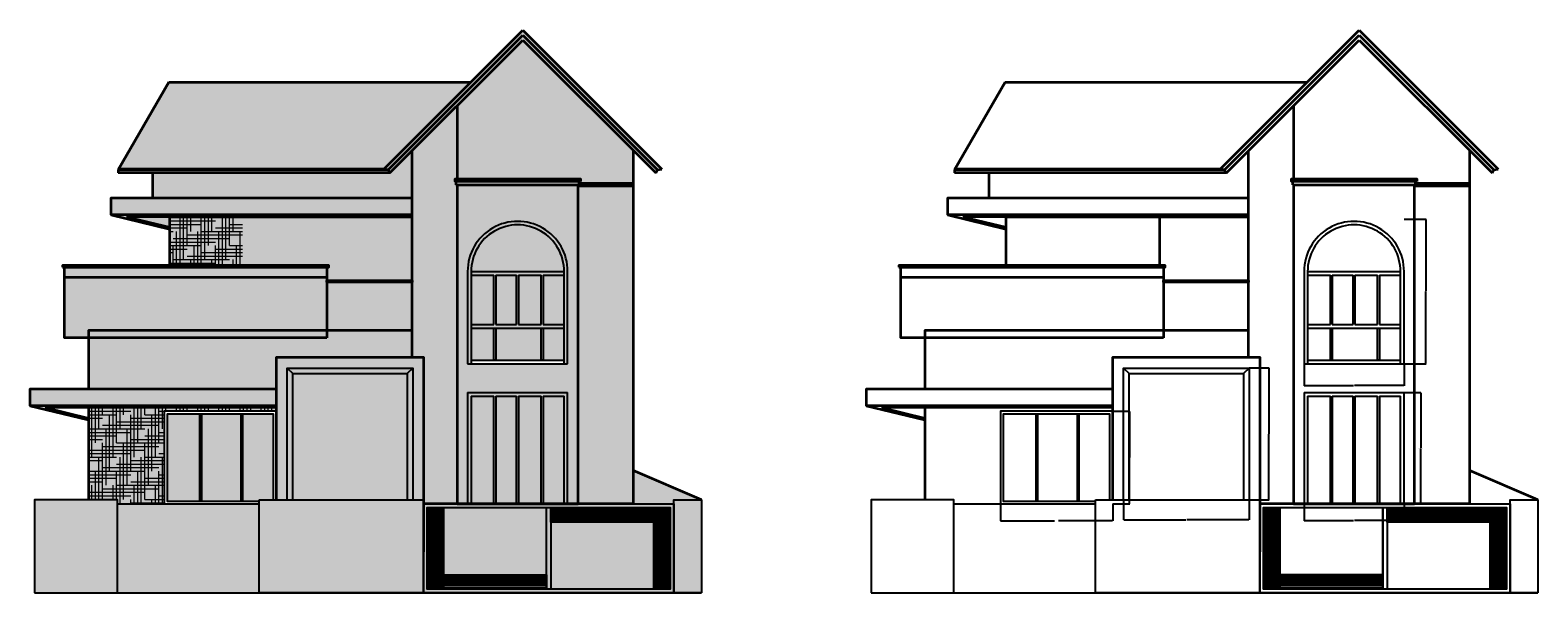
# Model space of a CAD drawing. Units: feet. Extents: x 2649 to 4006, y 754 to 1261.
import ezdxf

# ---------------------------------------------------------------- set-up
doc = ezdxf.new("R2010")
doc.units = ezdxf.units.FT
for name, color, linetype, lineweight in [('A-ANNO-DIMS', 2, 'Continuous', 18), ('A-DOOR', 3, 'Continuous', 25), ('A-ELEV', 7, 'Continuous', 35), ('A-ELEV-FENC', 8, 'Continuous', 25), ('A-ELEV-PATT', 8, 'Continuous', 13), ('A-GLAZ', 4, 'Continuous', 25), ('A-ROOF', 1, 'Continuous', 35)]:
    doc.layers.add(name, color=color, linetype=linetype, lineweight=lineweight)
doc.styles.get("Standard").update_dxf_attribs({"font": 'arial.ttf'})
doc.dimstyles.get("Standard").update_dxf_attribs({"dimtxt": 0.18, "dimasz": 0.18, "dimexe": 0.18, "dimexo": 0.0625, "dimgap": 0.09, "dimtad": 0, "dimtih": 1, "dimtoh": 1, "dimdec": 1, "dimzin": 0, "dimdsep": 46, "dimlunit": 3, "dimtxsty": 'Standard', "dimcen": 0.09, "dimadec": 0, "dimazin": 0, "dimtfac": 1, "dimtdec": 1, "dimtofl": 0, "dimtmove": 0, "dimatfit": 3, "dimfxl": 1, "dimtolj": 1, "dimtzin": 0, "dimarcsym": 0})

# ---------------------------------------------------------------- blocks, each defined once
blk = doc.blocks.new('WIN-ARCHED')
for p, q in [((3.2, 83.1), (86.8, 83.1)), ((3.2, 79.9), (23.7, 79.9)), ((25.4, 79.9), (44.1, 79.9)), ((45.8, 79.9), (66.2, 79.9)), ((67.9, 79.9), (86.8, 79.9)), ((3.2, 35.3), (23.7, 35.3)), ((3.2, 32.1), (86.8, 32.1)), ((25.4, 35.3), (44.1, 35.3)), ((45.8, 35.3), (66.2, 35.3)), ((67.9, 35.3), (86.8, 35.3)), ((0, 0), (90, 0)), ((3.2, 3.2), (86.8, 3.2))]:
    blk.add_line(p, q)
for points in [[(0, 83.4), (0, 0)], [(3.2, 83.5), (3.2, 0)], [(86.8, 0), (86.8, 83.5)], [(90, 0), (90, 83.4)], [(23.7, 35.3), (23.7, 79.9)], [(25.4, 79.9), (25.4, 35.3)], [(44.1, 35.3), (44.1, 79.9)], [(45.8, 79.9), (45.8, 35.3)], [(66.2, 35.3), (66.2, 79.9)], [(67.9, 79.9), (67.9, 35.3)], [(25.4, 32.1), (25.4, 3.2), (23.7, 3.2), (23.7, 32.1)], [(67.9, 32.1), (67.9, 3.2), (66.2, 3.2), (66.2, 32.1)]]:
    blk.add_lwpolyline(points)
for radius, start, end in [(45, 359.816, 180.184), (41.8, 359.7048, 180.2952)]:
    blk.add_arc((45, 83.3), radius, start, end)
blk = doc.blocks.new('DOOR-GLAZED-FRENCH')
for points in [[(0, 100.3), (90, 100.3)], [(0, 100.3), (0, 0)], [(3.2, 97.1), (3.2, 0)], [(3.2, 97.1), (23.7, 97.1)], [(25.4, 97.1), (25.4, 0), (23.7, 0), (23.7, 97.1)], [(25.4, 97.1), (44.1, 97.1)], [(45.8, 97.1), (45.8, 0), (44.1, 0), (44.1, 97.1)], [(45.8, 97.1), (66.2, 97.1)], [(67.9, 97.1), (67.9, 0), (66.2, 0), (66.2, 97.1)], [(67.9, 97.1), (86.8, 97.1)], [(86.8, 0), (86.8, 97.1)], [(90, 0), (90, 100.3)], [(90, 0), (0, 0)]]:
    blk.add_lwpolyline(points)
blk = doc.blocks.new('WIN-SLIDING')
for points in [[(101, 3.6), (101, 83.4), (0, 83.4), (0, 0), (85.6, 0)], [(98.4, 3.6), (98.4, 80.8), (2.6, 80.8), (2.6, 2.6), (85.6, 2.6)]]:
    blk.add_lwpolyline(points)
for points in [[(32.2, 80.8), (33.5, 80.8), (33.5, 2.6), (32.2, 2.6)], [(69.3, 80.8), (70.6, 80.8), (70.6, 2.6), (69.3, 2.6)]]:
    blk.add_lwpolyline(points, close=True)
blk = doc.blocks.new('DOOR-MAIN')
for p, q in [((0, 118.8), (5, 113.8)), ((113, 118.8), (108, 113.8))]:
    blk.add_line(p, q)
for points in [[(0, 0), (0, 118.8), (113, 118.8), (113, 0)], [(5, 0), (5, 113.8), (108, 113.8), (108, 0)]]:
    blk.add_lwpolyline(points)
blk = doc.blocks.new('*D5')
at = {"layer": 'A-ANNO-DIMS', "color": 0, "lineweight": -2, "transparency": 16777216}
for p, q in [((3885.8, 1090.6), (3905.5, 1090.6)), ((3905.3, 1090.4), (3905.3, 1025.6)), ((3905.3, 960.5), (3905.3, 1025.2)), ((3885.8, 960.3), (3905.5, 960.3))]:
    blk.add_line(p, q, dxfattribs=at)
at = {"layer": 'A-ANNO-DIMS', "color": 0, "transparency": 16777216}
for points in [[(3905.3, 1090.4), (3905.3, 1090.4), (3905.3, 1090.6)], [(3905.3, 960.5), (3905.3, 960.5), (3905.3, 960.3)]]:
    blk.add_solid(points, dxfattribs=at)
at = {"layer": 'Defpoints', "color": 0, "transparency": 16777216}
for p in [(3885.8, 1090.6), (3905.3, 1090.6), (3885.8, 960.3)]:
    blk.add_point(p, dxfattribs=at)
at = {"layer": 'A-ANNO-DIMS', "color": 0, "transparency": 16777216, "insert": (3905.3, 1025.4), "char_height": 0.18, "attachment_point": 5}
blk.add_mtext('\\A1;ARCHED WINDOW 130 TYP.', dxfattribs=at)
blk = doc.blocks.new('*D6')
at = {"layer": 'A-ANNO-DIMS', "color": 0, "lineweight": -2, "transparency": 16777216}
for p, q in [((3795.7, 960.2), (3795.7, 940.5)), ((3885.8, 960.2), (3885.8, 940.5)), ((3795.9, 940.7), (3840.2, 940.7)), ((3885.6, 940.7), (3841.2, 940.7))]:
    blk.add_line(p, q, dxfattribs=at)
at = {"layer": 'A-ANNO-DIMS', "color": 0, "transparency": 16777216}
for points in [[(3795.9, 940.8), (3795.9, 940.7), (3795.7, 940.7)], [(3885.6, 940.8), (3885.6, 940.7), (3885.8, 940.7)]]:
    blk.add_solid(points, dxfattribs=at)
at = {"layer": 'Defpoints', "color": 0, "transparency": 16777216}
for p in [(3795.7, 960.3), (3885.8, 960.3), (3885.8, 940.7)]:
    blk.add_point(p, dxfattribs=at)
at = {"layer": 'A-ANNO-DIMS', "color": 0, "transparency": 16777216, "insert": (3840.7, 940.7), "char_height": 0.18, "attachment_point": 5}
blk.add_mtext('\\A1;90 TYP.', dxfattribs=at)
blk = doc.blocks.new('*D7')
at = {"layer": 'A-ANNO-DIMS', "color": 0, "lineweight": -2, "transparency": 16777216}
for p, q in [((3885.8, 934.4), (3900.9, 934.4)), ((3900.8, 934.2), (3900.8, 884.5)), ((3900.8, 834.3), (3900.8, 884.1)), ((3885.8, 834.1), (3900.9, 834.1))]:
    blk.add_line(p, q, dxfattribs=at)
at = {"layer": 'A-ANNO-DIMS', "color": 0, "transparency": 16777216}
for points in [[(3900.7, 934.2), (3900.8, 934.2), (3900.8, 934.4)], [(3900.7, 834.3), (3900.8, 834.3), (3900.8, 834.1)]]:
    blk.add_solid(points, dxfattribs=at)
at = {"layer": 'Defpoints', "color": 0, "transparency": 16777216}
for p in [(3885.7, 934.4), (3900.8, 934.4), (3885.7, 834.1)]:
    blk.add_point(p, dxfattribs=at)
at = {"layer": 'A-ANNO-DIMS', "color": 0, "transparency": 16777216, "insert": (3900.8, 884.3), "char_height": 0.18, "attachment_point": 5}
blk.add_mtext('\\A1;GLAZED FRENCH DOOR 100 TYP.', dxfattribs=at)
blk = doc.blocks.new('*D8')
at = {"layer": 'A-ANNO-DIMS', "color": 0, "lineweight": -2, "transparency": 16777216}
for p, q in [((3795.7, 834.1), (3795.7, 818.9)), ((3885.7, 834.1), (3885.7, 818.9)), ((3795.9, 819.1), (3840.2, 819.1)), ((3885.5, 819.1), (3841.2, 819.1))]:
    blk.add_line(p, q, dxfattribs=at)
at = {"layer": 'A-ANNO-DIMS', "color": 0, "transparency": 16777216}
for points in [[(3795.9, 819.1), (3795.9, 819.1), (3795.7, 819.1)], [(3885.5, 819.1), (3885.5, 819.1), (3885.7, 819.1)]]:
    blk.add_solid(points, dxfattribs=at)
at = {"layer": 'Defpoints', "color": 0, "transparency": 16777216}
for p in [(3795.7, 834.1), (3885.7, 834.1), (3885.7, 819.1)]:
    blk.add_point(p, dxfattribs=at)
at = {"layer": 'A-ANNO-DIMS', "color": 0, "transparency": 16777216, "insert": (3840.7, 819.1), "char_height": 0.18, "attachment_point": 5}
blk.add_mtext('\\A1;90 TYP.', dxfattribs=at)
blk = doc.blocks.new('*D9')
at = {"layer": 'A-ANNO-DIMS', "color": 0, "lineweight": -2, "transparency": 16777216}
for p, q in [((3522.5, 834.1), (3522.5, 818.8)), ((3623.6, 834.1), (3623.6, 818.8)), ((3522.7, 819), (3571.3, 819)), ((3623.4, 819), (3574.8, 819))]:
    blk.add_line(p, q, dxfattribs=at)
at = {"layer": 'A-ANNO-DIMS', "color": 0, "transparency": 16777216}
for points in [[(3522.7, 819), (3522.7, 818.9), (3522.5, 819)], [(3623.4, 819), (3623.4, 818.9), (3623.6, 819)]]:
    blk.add_solid(points, dxfattribs=at)
at = {"layer": 'Defpoints', "color": 0, "transparency": 16777216}
for p in [(3522.5, 834.1), (3623.6, 834.1), (3623.6, 819)]:
    blk.add_point(p, dxfattribs=at)
at = {"layer": 'A-ANNO-DIMS', "color": 0, "transparency": 16777216, "insert": (3573, 819), "char_height": 0.18, "attachment_point": 5}
blk.add_mtext('\\A1;SLIDING WINDOW 101 TYP.', dxfattribs=at)
blk = doc.blocks.new('*D10')
at = {"layer": 'A-ANNO-DIMS', "color": 0, "lineweight": -2, "transparency": 16777216}
for p, q in [((3623.6, 917.5), (3638.9, 917.5)), ((3638.7, 917.3), (3638.7, 876)), ((3638.7, 834.3), (3638.7, 875.6)), ((3623.6, 834.1), (3638.9, 834.1))]:
    blk.add_line(p, q, dxfattribs=at)
at = {"layer": 'A-ANNO-DIMS', "color": 0, "transparency": 16777216}
for points in [[(3638.7, 917.3), (3638.7, 917.3), (3638.7, 917.5)], [(3638.7, 834.3), (3638.7, 834.3), (3638.7, 834.1)]]:
    blk.add_solid(points, dxfattribs=at)
at = {"layer": 'Defpoints', "color": 0, "transparency": 16777216}
for p in [(3623.6, 917.5), (3638.7, 917.5), (3623.6, 834.1)]:
    blk.add_point(p, dxfattribs=at)
at = {"layer": 'A-ANNO-DIMS', "color": 0, "transparency": 16777216, "insert": (3638.7, 875.8), "char_height": 0.18, "attachment_point": 5}
blk.add_mtext('\\A1;83 TYP.', dxfattribs=at)
blk = doc.blocks.new('*D11')
at = {"layer": 'A-ANNO-DIMS', "color": 0, "lineweight": -2, "transparency": 16777216}
for p, q in [((3746.3, 956.6), (3764.3, 956.6)), ((3764.1, 956.4), (3764.1, 897.3)), ((3764.1, 837.9), (3764.1, 897)), ((3746.3, 837.7), (3764.3, 837.7))]:
    blk.add_line(p, q, dxfattribs=at)
at = {"layer": 'A-ANNO-DIMS', "color": 0, "transparency": 16777216}
for points in [[(3764.1, 956.4), (3764.1, 956.4), (3764.1, 956.6)], [(3764.1, 837.9), (3764.1, 837.9), (3764.1, 837.7)]]:
    blk.add_solid(points, dxfattribs=at)
at = {"layer": 'Defpoints', "color": 0, "transparency": 16777216}
for p in [(3746.3, 956.6), (3764.1, 956.6), (3746.3, 837.7)]:
    blk.add_point(p, dxfattribs=at)
at = {"layer": 'A-ANNO-DIMS', "color": 0, "transparency": 16777216, "insert": (3764.1, 897.2), "char_height": 0.18, "attachment_point": 5}
blk.add_mtext('\\A1;MAIN DOOR 119 TYP.', dxfattribs=at)
blk = doc.blocks.new('*D12')
at = {"layer": 'A-ANNO-DIMS', "color": 0, "lineweight": -2, "transparency": 16777216}
for p, q in [((3633.2, 837.7), (3633.2, 819.7)), ((3746.3, 837.7), (3746.3, 819.7)), ((3633.4, 819.9), (3689.2, 819.9)), ((3746.1, 819.9), (3690.3, 819.9))]:
    blk.add_line(p, q, dxfattribs=at)
at = {"layer": 'A-ANNO-DIMS', "color": 0, "transparency": 16777216}
for points in [[(3633.4, 820), (3633.4, 819.9), (3633.2, 819.9)], [(3746.1, 820), (3746.1, 819.9), (3746.3, 819.9)]]:
    blk.add_solid(points, dxfattribs=at)
at = {"layer": 'Defpoints', "color": 0, "transparency": 16777216}
for p in [(3633.2, 837.7), (3746.3, 837.7), (3746.3, 819.9)]:
    blk.add_point(p, dxfattribs=at)
at = {"layer": 'A-ANNO-DIMS', "color": 0, "transparency": 16777216, "insert": (3689.8, 819.9), "char_height": 0.18, "attachment_point": 5}
blk.add_mtext('\\A1;113 TYP.', dxfattribs=at)

msp = doc.modelspace()

# ---------------------------------------------------------------- hatches: boundary and pattern name
at = {"layer": 'A-ELEV-PATT'}
h = msp.add_hatch(color=256, dxfattribs=at)
h.dxf.hatch_style = 1
h.paths.add_polyline_path([(3045.9, 1214), (2774.1, 1214), (2728.9, 1135.7), (2967.7, 1135.7)])
h.paths.add_polyline_path([(2967.7, 1135.7), (2728.9, 1135.7), (2728.6, 1135.1), (2971.6, 1135.1)])
h.paths.add_polyline_path([(2971.6, 1135.1), (2728.6, 1135.1), (2728.6, 1132.2), (2973.2, 1132.2)])
h.paths.add_polyline_path([(3092.8, 1256.3), (3213.9, 1135.1), (3217.8, 1135.7), (3092.8, 1260.8), (2967.7, 1135.7), (2971.6, 1135.1)])
h.paths.add_polyline_path([(3092.8, 1251.7), (3212.3, 1132.2), (3213.9, 1135.1), (3092.8, 1256.3), (2971.6, 1135.1), (2973.2, 1132.2)])
h.paths.add_polyline_path([(2993.1, 1109.8), (2759.7, 1109.8), (2722.5, 1109.8), (2722.5, 1094.4), (2993.1, 1094.4)])
h.paths.add_polyline_path([(2871, 937.8), (2701.9, 937.8), (2649.5, 937.8), (2649.5, 922.4), (2871, 922.4)])
h = msp.add_hatch(color=256, dxfattribs=at)
h.dxf.hatch_style = 1
h.paths.add_polyline_path([(3092.8, 1251.7), (3033.7, 1192.6), (3033.7, 1126.8), (3144.6, 1126.8), (3144.6, 1124.6), (3143.5, 1124.6), (3143.5, 1122.8), (3191.9, 1122.8), (3191.9, 1152.6)])
h.paths.add_polyline_path([(3191.9, 1120.2), (3142.6, 1120.2), (3142.6, 834.1), (3191.9, 834.1)])
h.paths.add_polyline_path([(3109.4, 1040.2), (3109.4, 995.6), (3089, 995.6), (3089, 1040.2)], flags=0)
h.paths.add_polyline_path([(3087.3, 1040.2), (3087.3, 995.6), (3068.6, 995.6), (3068.6, 1040.2)], flags=0)
h.paths.add_polyline_path([(3111.1, 992.4), (3111.1, 963.5), (3109.4, 963.5), (3109.4, 992.4), (3068.6, 992.4), (3068.6, 963.5), (3066.9, 963.5), (3066.9, 992.4)], flags=0)
h = msp.add_hatch(color=256, dxfattribs=at)
h.dxf.hatch_style = 1
h.paths.add_polyline_path([(3033.7, 1121.4), (3032.6, 1121.4), (3032.6, 1124.6), (3031.8, 1124.6), (3031.8, 1126.8), (3033.7, 1126.8), (3033.7, 1192.6), (2993.1, 1152), (2993.1, 966.3), (3003.4, 966.3), (3003.4, 834.1), (3033.7, 834.1)])
h.paths.add_polyline_path([(2993.1, 1092.8), (2913.5, 1092.8), (2913.5, 1048.8), (2918.1, 1048.8), (2918.1, 1047.2), (2916.5, 1047.2), (2916.5, 1035.2), (2993.1, 1035.2)])
h.paths.add_polyline_path([(3003.4, 966.3), (2993.1, 966.3), (2871, 966.3), (2871, 837.7), (2880.7, 837.7), (2880.7, 956.6), (2993.7, 956.6), (2993.7, 837.7), (3003.4, 837.7)])
h.paths.add_polyline_path([(2993.7, 956.6), (2988.6, 951.5), (2988.6, 837.7), (2993.7, 837.7)], flags=17)
h.paths.add_polyline_path([(2993.7, 956.6), (2880.7, 956.6), (2885.7, 951.5), (2988.6, 951.5)], flags=17)
h.paths.add_polyline_path([(2885.7, 951.5), (2880.7, 956.6), (2880.7, 837.7), (2885.7, 837.7)], flags=17)
h.paths.add_polyline_path([(3210.5, 817.8), (3118, 817.8), (3118, 757.2), (3210.5, 757.2)])
h.paths.add_polyline_path([(2855.5, 834.1), (2770, 834.1), (2728.1, 834.1), (2728.1, 754), (2855.5, 754)])
h.paths.add_polyline_path([(2988.6, 951.5), (2885.7, 951.5), (2885.7, 837.7), (2988.6, 837.7)], flags=17)
h.paths.add_polyline_path([(2775, 1092.8), (2736, 1092.8), (2775, 1083.3)])
h = msp.add_hatch(color=256, dxfattribs=at)
h.dxf.hatch_style = 1
h.paths.add_polyline_path([(2993.1, 1152), (2973.2, 1132.2), (2759.7, 1132.2), (2759.7, 1109.8), (2993.1, 1109.8)])
h = msp.add_hatch(color=256, dxfattribs=at)
h.dxf.hatch_style = 1
h.paths.add_polyline_path([(2916.5, 1038.2), (2680.4, 1038.2), (2680.4, 983.6), (2701.9, 983.6), (2701.9, 990.4), (2916.5, 990.4)])
h.paths.add_polyline_path([(2916.5, 1047.2), (2680.4, 1047.2), (2680.4, 1038.2), (2916.5, 1038.2)])
h.paths.add_polyline_path([(2918.1, 1048.8), (2678.6, 1048.8), (2678.6, 1047.2), (2918.1, 1047.2)])
h.paths.add_polyline_path([(2916.5, 990.4), (2701.9, 990.4), (2701.9, 983.6), (2916.5, 983.6)], flags=17)
h.paths.add_polyline_path([(2728.1, 837.7), (2653.5, 837.7), (2653.5, 754), (2728.1, 754)])
h.paths.add_polyline_path([(3003.4, 837.7), (2855.5, 837.7), (2855.5, 754), (3003.4, 754), (3003.4, 834.1)])
h.paths.add_polyline_path([(3253.5, 837.7), (3228.6, 837.7), (3228.6, 754), (3253.5, 754)])
h.paths.add_polyline_path([(3191.9, 864.2), (3191.9, 834.1), (3228.6, 834.1), (3228.6, 837.7), (3253.5, 837.7)])
h.paths.add_polyline_path([(3143.5, 1124.6), (3032.6, 1124.6), (3032.6, 1121.4), (3143.5, 1121.4)])
h.paths.add_polyline_path([(3144.6, 1126.8), (3031.8, 1126.8), (3031.8, 1124.6), (3144.6, 1124.6)])
h.paths.add_polyline_path([(3192.4, 1122.8), (3143.5, 1122.8), (3143.5, 1121.4), (3142.6, 1121.4), (3142.6, 1121), (3192.4, 1121)])
h.paths.add_polyline_path([(3142.6, 1121.4), (3033.7, 1121.4), (3033.7, 834.1), (3043.2, 834.1), (3043.2, 934.4), (3133.1, 934.4), (3133.1, 834.1), (3142.6, 834.1)])
h.paths.add_polyline_path([(3133.1, 960.3), (3043.2, 960.3), (3043.2, 1043.4, -1.003216), (3133.1, 1043.4)], flags=16)
h.paths.add_polyline_path([(3130, 963.5), (3046.3, 963.5), (3046.3, 1043.3, -1.005166), (3130, 1043.3)], flags=0)
h.paths.add_polyline_path([(3111.1, 963.5), (3109.4, 963.5), (3109.4, 992.4), (3068.6, 992.4), (3068.6, 963.5), (3066.9, 963.5), (3066.9, 992.4), (3111.1, 992.4)], flags=0)
h.paths.add_polyline_path([(3109.4, 995.6), (3089, 995.6), (3089, 1040.2), (3109.4, 1040.2)], flags=0)
h.paths.add_polyline_path([(3087.3, 995.6), (3068.6, 995.6), (3068.6, 1040.2), (3087.3, 1040.2)], flags=0)
h.paths.add_polyline_path([(3046.3, 1043.3, -1.005166), (3130, 1043.3), (3130, 960.3), (3133.1, 960.3), (3133.1, 1043.7, 0.996794), (3043.2, 1043.7), (3043.2, 960.3), (3046.3, 960.3)], flags=16)
h.paths.add_polyline_path([(3130, 963.5), (3046.3, 963.5), (3046.3, 960.3), (3130, 960.3)], flags=0)
h = msp.add_hatch(color=256, dxfattribs=at)
h.dxf.hatch_style = 1
h.paths.add_polyline_path([(2993.1, 1094.4), (2722.5, 1094.4), (2775, 1081.7), (2775, 1083.3), (2736, 1092.8), (2993.1, 1092.8)])
h.paths.add_polyline_path([(2871, 922.4), (2649.5, 922.4), (2701.9, 909.7), (2701.9, 911.3), (2663, 920.8), (2871, 920.8)])
h = msp.add_hatch(color=256, dxfattribs=at)
h.dxf.hatch_style = 1
h.paths.add_polyline_path([(2913.5, 1092.8), (2840.6, 1092.8), (2840.6, 1048.8), (2913.5, 1048.8)])
h.paths.add_polyline_path([(2840.6, 1092.8), (2775, 1092.8), (2775, 1048.8), (2840.6, 1048.8)])
h.paths.add_polyline_path([(2770, 917.5), (2871, 917.5), (2871, 920.8), (2701.9, 920.8), (2701.9, 837.7), (2728.1, 837.7), (2728.1, 834.1), (2770, 834.1)])
h = msp.add_hatch(dxfattribs=at)
h.set_pattern_fill('HOUND', color=256, scale=2)
h.set_pattern_definition([(0, (-752.5737, 0), (12.7, 3.175), [50.8, -25.4]), (90, (-752.5737, 0), (-3.175, -12.7), [50.8, -25.4])])
h.paths.add_polyline_path([(2840.6, 1092.8), (2775, 1092.8), (2775, 1048.8), (2840.6, 1048.8)])
h.paths.add_polyline_path([(2770, 917.5), (2871, 917.5), (2871, 920.8), (2701.9, 920.8), (2701.9, 837.7), (2728.1, 837.7), (2728.1, 834.1), (2770, 834.1)])
h = msp.add_hatch(color=256, dxfattribs=at)
h.dxf.hatch_style = 1
h.paths.add_polyline_path([(3046.3, 1043.8), (3046.3, 1043.3), (3130, 1043.3), (3130, 1043.8, 0.994861)])
h.paths.add_polyline_path([(3066.9, 1040.2), (3046.3, 1040.2), (3046.3, 995.6), (3066.9, 995.6)])
h.paths.add_polyline_path([(3087.3, 1040.2), (3068.6, 1040.2), (3068.6, 995.6), (3087.3, 995.6)])
h.paths.add_polyline_path([(3130, 1040.2), (3111.1, 1040.2), (3111.1, 995.6), (3130, 995.6)])
h.paths.add_polyline_path([(3109.4, 1040.2), (3089, 1040.2), (3089, 995.6), (3109.4, 995.6)])
h.paths.add_polyline_path([(3109.4, 992.4), (3068.6, 992.4), (3068.6, 963.5), (3109.4, 963.5)])
h.paths.add_polyline_path([(3130, 992.4), (3111.1, 992.4), (3111.1, 963.5), (3130, 963.5)])
h.paths.add_polyline_path([(3066.9, 992.4), (3046.3, 992.4), (3046.3, 963.5), (3066.9, 963.5)])
h.paths.add_polyline_path([(3066.9, 931.2), (3046.3, 931.2), (3046.3, 834.1), (3066.9, 834.1)])
h.paths.add_polyline_path([(3087.3, 931.2), (3068.6, 931.2), (3068.6, 834.1), (3087.3, 834.1)])
h.paths.add_polyline_path([(3109.4, 931.2), (3089, 931.2), (3089, 834.1), (3109.4, 834.1)])
h.paths.add_polyline_path([(3130, 931.2), (3111.1, 931.2), (3111.1, 834.1), (3130, 834.1)])
h.paths.add_polyline_path([(2802.2, 914.9), (2772.6, 914.9), (2772.6, 836.7), (2802.2, 836.7)])
h.paths.add_polyline_path([(2839.3, 914.9), (2803.5, 914.9), (2803.5, 836.7), (2839.3, 836.7)])
h.paths.add_polyline_path([(2868.4, 914.9), (2840.6, 914.9), (2840.6, 836.7), (2855.5, 836.7), (2855.5, 837.7), (2868.4, 837.7)])
h.paths.add_polyline_path([(2993.1, 1033.7), (2916.5, 1033.7), (2916.5, 990.4), (2993.1, 990.4)])
h = msp.add_hatch(color=256, dxfattribs=at)
h.dxf.hatch_style = 1
h.paths.add_polyline_path([(3130, 1043.3), (3046.3, 1043.3), (3046.3, 1040.2), (3066.9, 1040.2), (3066.9, 995.6), (3046.3, 995.6), (3046.3, 992.4), (3130, 992.4), (3130, 995.6), (3111.1, 995.6), (3111.1, 1040.2), (3130, 1040.2)])
h.paths.add_polyline_path([(3087.3, 1040.2), (3087.3, 995.6), (3068.6, 995.6), (3068.6, 1040.2)], flags=16)
h.paths.add_polyline_path([(3089, 1040.2), (3109.4, 1040.2), (3109.4, 995.6), (3089, 995.6)], flags=16)
h.paths.add_polyline_path([(3068.6, 992.4), (3066.9, 992.4), (3066.9, 963.5), (3068.6, 963.5)])
h.paths.add_polyline_path([(3111.1, 992.4), (3109.4, 992.4), (3109.4, 963.5), (3111.1, 963.5)])
h = msp.add_hatch(color=256, dxfattribs=at)
h.dxf.hatch_style = 1
h.paths.add_polyline_path([(2993.1, 990.4), (2916.5, 990.4), (2916.5, 983.6), (2701.9, 983.6), (2701.9, 937.8), (2871, 937.8), (2871, 966.3), (2993.1, 966.3)])
h = msp.add_hatch(color=256, dxfattribs=at)
h.dxf.hatch_style = 1
h.paths.add_polyline_path([(3133.1, 934.4), (3043.2, 934.4), (3043.2, 834.1), (3046.3, 834.1), (3046.3, 931.2), (3066.9, 931.2), (3066.9, 834.1), (3068.6, 834.1), (3068.6, 931.2), (3087.3, 931.2), (3087.3, 834.1), (3089, 834.1), (3089, 931.2), (3109.4, 931.2), (3109.4, 834.1), (3111.1, 834.1), (3111.1, 931.2), (3130, 931.2), (3130, 834.1), (3133.1, 834.1)])
h = msp.add_hatch(color=256, dxfattribs=at)
h.dxf.hatch_style = 1
h.paths.add_polyline_path([(3228.6, 834.1), (3003.4, 834.1), (3003.4, 791), (3003.4, 754), (3228.6, 754)])
h.paths.add_polyline_path([(3020.4, 830.9), (3021.4, 830.9), (3114, 830.9), (3118, 830.9), (3210.5, 830.9), (3211.6, 830.9), (3225.3, 830.9), (3225.3, 757.2), (3211.6, 757.2), (3210.5, 757.2), (3006.6, 757.2), (3006.6, 830.9)], flags=16)
h.paths.add_polyline_path([(3007.7, 830.9), (3007.7, 757.2), (3007.3, 757.2), (3007.3, 830.9)], flags=0)
h.paths.add_polyline_path([(3008.8, 830.9), (3009.3, 830.9), (3009.3, 757.2), (3008.8, 757.2)], flags=0)
h.paths.add_polyline_path([(3010.3, 830.9), (3010.8, 830.9), (3010.8, 757.2), (3010.3, 757.2)], flags=0)
h.paths.add_polyline_path([(3011.9, 830.9), (3012.3, 830.9), (3012.3, 757.2), (3011.9, 757.2)], flags=0)
h.paths.add_polyline_path([(3013.4, 830.9), (3013.9, 830.9), (3013.9, 757.2), (3013.4, 757.2)], flags=0)
h.paths.add_polyline_path([(3014.9, 830.9), (3015.4, 830.9), (3015.4, 757.2), (3014.9, 757.2)], flags=0)
h.paths.add_polyline_path([(3016.5, 830.9), (3016.9, 830.9), (3016.9, 757.2), (3016.5, 757.2)], flags=0)
h.paths.add_polyline_path([(3018, 830.9), (3018.5, 830.9), (3018.5, 757.2), (3018, 757.2)], flags=0)
h.paths.add_polyline_path([(3019.6, 830.9), (3020, 830.9), (3020, 757.2), (3019.6, 757.2)], flags=0)
h.paths.add_polyline_path([(3021.4, 770.3), (3114, 770.3), (3114, 757.2), (3021.4, 757.2)], flags=0)
h.paths.add_polyline_path([(3021.4, 769.2), (3114, 769.2), (3114, 768.7), (3021.4, 768.7)], flags=0)
h.paths.add_polyline_path([(3021.4, 767.1), (3114, 767.1), (3114, 766.5), (3021.4, 766.5)], flags=0)
h.paths.add_polyline_path([(3021.4, 765), (3114, 765), (3114, 764.4), (3021.4, 764.4)], flags=0)
h.paths.add_polyline_path([(3021.4, 762.9), (3114, 762.9), (3114, 762.3), (3021.4, 762.3)], flags=0)
h.paths.add_polyline_path([(3021.4, 760.8), (3114, 760.8), (3114, 760.2), (3021.4, 760.2)], flags=0)
h.paths.add_polyline_path([(3021.4, 758.6), (3114, 758.6), (3114, 758.1), (3021.4, 758.1)], flags=0)
h.paths.add_polyline_path([(3118, 830.2), (3210.5, 830.2), (3210.5, 829.6), (3118, 829.6)], flags=0)
h.paths.add_polyline_path([(3118, 828.3), (3210.5, 828.3), (3210.5, 827.8), (3118, 827.8)], flags=0)
h.paths.add_polyline_path([(3118, 826.5), (3210.5, 826.5), (3210.5, 825.9), (3118, 825.9)], flags=0)
h.paths.add_polyline_path([(3118, 824.6), (3210.5, 824.6), (3210.5, 824), (3118, 824)], flags=0)
h.paths.add_polyline_path([(3118, 822.7), (3210.5, 822.7), (3210.5, 822.1), (3118, 822.1)], flags=0)
h.paths.add_polyline_path([(3118, 820.8), (3210.5, 820.8), (3210.5, 820.3), (3118, 820.3)], flags=0)
h.paths.add_polyline_path([(3118, 819), (3210.5, 819), (3210.5, 818.4), (3118, 818.4)], flags=0)
h.paths.add_polyline_path([(3211.9, 830.9), (3212.4, 830.9), (3212.4, 757.2), (3211.9, 757.2)], flags=0)
h.paths.add_polyline_path([(3213.5, 830.9), (3213.9, 830.9), (3213.9, 757.2), (3213.5, 757.2)], flags=0)
h.paths.add_polyline_path([(3215, 830.9), (3215.5, 830.9), (3215.5, 757.2), (3215, 757.2)], flags=0)
h.paths.add_polyline_path([(3216.5, 830.9), (3217, 830.9), (3217, 757.2), (3216.5, 757.2)], flags=0)
h.paths.add_polyline_path([(3218.1, 830.9), (3218.5, 830.9), (3218.5, 757.2), (3218.1, 757.2)], flags=0)
h.paths.add_polyline_path([(3219.6, 830.9), (3220.1, 830.9), (3220.1, 757.2), (3219.6, 757.2)], flags=0)
h.paths.add_polyline_path([(3221.1, 830.9), (3221.6, 830.9), (3221.6, 757.2), (3221.1, 757.2)], flags=0)
h.paths.add_polyline_path([(3222.7, 830.9), (3223.2, 830.9), (3223.2, 757.2), (3222.7, 757.2)], flags=0)
h.paths.add_polyline_path([(3224.2, 830.9), (3224.7, 830.9), (3224.7, 757.2), (3224.2, 757.2)], flags=0)
h = msp.add_hatch(color=256, dxfattribs=at)
h.dxf.hatch_style = 1
h.paths.add_polyline_path([(3007.7, 830.9), (3007.3, 830.9), (3007.3, 757.2), (3007.7, 757.2)])
h.paths.add_polyline_path([(3009.3, 830.9), (3008.8, 830.9), (3008.8, 757.2), (3009.3, 757.2)])
h.paths.add_polyline_path([(3010.8, 830.9), (3010.3, 830.9), (3010.3, 757.2), (3010.8, 757.2)])
h.paths.add_polyline_path([(3012.3, 830.9), (3011.9, 830.9), (3011.9, 757.2), (3012.3, 757.2)])
h.paths.add_polyline_path([(3013.9, 830.9), (3013.4, 830.9), (3013.4, 757.2), (3013.9, 757.2)])
h.paths.add_polyline_path([(3015.4, 830.9), (3014.9, 830.9), (3014.9, 757.2), (3015.4, 757.2)])
h.paths.add_polyline_path([(3016.9, 830.9), (3016.5, 830.9), (3016.5, 757.2), (3016.9, 757.2)])
h.paths.add_polyline_path([(3018.5, 830.9), (3018, 830.9), (3018, 757.2), (3018.5, 757.2)])
h.paths.add_polyline_path([(3020, 830.9), (3019.6, 830.9), (3019.6, 757.2), (3020, 757.2)])
h = msp.add_hatch(color=256, dxfattribs=at)
h.dxf.hatch_style = 1
h.paths.add_polyline_path([(3114, 830.9), (3021.4, 830.9), (3021.4, 770.3), (3114, 770.3)])
h = msp.add_hatch(color=256, dxfattribs=at)
h.dxf.hatch_style = 1
h.paths.add_polyline_path([(3114, 769.2), (3021.4, 769.2), (3021.4, 768.7), (3114, 768.7)])
h.paths.add_polyline_path([(3114, 767.1), (3021.4, 767.1), (3021.4, 766.5), (3114, 766.5)])
h.paths.add_polyline_path([(3114, 765), (3021.4, 765), (3021.4, 764.4), (3114, 764.4)])
h.paths.add_polyline_path([(3114, 762.9), (3021.4, 762.9), (3021.4, 762.3), (3114, 762.3)])
h.paths.add_polyline_path([(3114, 760.8), (3021.4, 760.8), (3021.4, 760.2), (3114, 760.2)])
h.paths.add_polyline_path([(3118, 830.9), (3114, 830.9), (3114, 770.3), (3114, 757.2), (3118, 757.2)])
h.paths.add_polyline_path([(3021.4, 758.1), (3114, 758.1), (3114, 758.6), (3021.4, 758.6)])
h = msp.add_hatch(color=256, dxfattribs=at)
h.dxf.hatch_style = 1
h.paths.add_polyline_path([(3210.5, 830.2), (3118, 830.2), (3118, 829.6), (3210.5, 829.6)])
h.paths.add_polyline_path([(3210.5, 828.3), (3118, 828.3), (3118, 827.8), (3210.5, 827.8)])
h.paths.add_polyline_path([(3210.5, 826.5), (3118, 826.5), (3118, 825.9), (3210.5, 825.9)])
h.paths.add_polyline_path([(3210.5, 824.6), (3118, 824.6), (3118, 824), (3210.5, 824)])
h.paths.add_polyline_path([(3210.5, 822.7), (3118, 822.7), (3118, 822.1), (3210.5, 822.1)])
h.paths.add_polyline_path([(3210.5, 820.8), (3118, 820.8), (3118, 820.3), (3210.5, 820.3)])
h.paths.add_polyline_path([(3210.5, 819), (3118, 819), (3118, 818.4), (3210.5, 818.4)])
h = msp.add_hatch(color=256, dxfattribs=at)
h.dxf.hatch_style = 1
h.paths.add_polyline_path([(3224.7, 830.9), (3224.2, 830.9), (3224.2, 757.2), (3224.7, 757.2)])
h.paths.add_polyline_path([(3223.2, 830.9), (3222.7, 830.9), (3222.7, 757.2), (3223.2, 757.2)])
h.paths.add_polyline_path([(3221.6, 830.9), (3221.1, 830.9), (3221.1, 757.2), (3221.6, 757.2)])
h.paths.add_polyline_path([(3220.1, 830.9), (3219.6, 830.9), (3219.6, 757.2), (3220.1, 757.2)])
h.paths.add_polyline_path([(3218.5, 830.9), (3218.1, 830.9), (3218.1, 757.2), (3218.5, 757.2)])
h.paths.add_polyline_path([(3217, 830.9), (3216.5, 830.9), (3216.5, 757.2), (3217, 757.2)])
h.paths.add_polyline_path([(3215.5, 830.9), (3215, 830.9), (3215, 757.2), (3215.5, 757.2)])
h.paths.add_polyline_path([(3213.9, 830.9), (3213.5, 830.9), (3213.5, 757.2), (3213.9, 757.2)])
h.paths.add_polyline_path([(3212.4, 830.9), (3211.9, 830.9), (3211.9, 757.2), (3212.4, 757.2)])

# ---------------------------------------------------------------- linework, layer by layer
at = {"layer": 'A-ELEV'}
for p, q in [((2759.7, 1109.8), (2759.7, 1132.2)), ((3512.3, 1109.8), (3512.3, 1132.2)), ((2722.5, 1094.4), (2775, 1081.7)), ((2736, 1092.8), (2775, 1083.3)), ((2993.1, 1092.8), (2736, 1092.8)), ((3475.1, 1094.4), (3527.6, 1081.7)), ((3488.6, 1092.8), (3527.6, 1083.3)), ((3745.6, 1092.8), (3488.6, 1092.8)), ((3666, 1048.8), (3666, 1092.8)), ((2680.4, 1038.2), (2916.5, 1038.2)), ((3432.9, 1038.2), (3669.1, 1038.2)), ((2649.5, 922.4), (2701.9, 909.7)), ((2663, 920.8), (2701.9, 911.3)), ((2871, 920.8), (2663, 920.8)), ((2701.9, 920.8), (2701.9, 837.7)), ((3402, 922.4), (3454.5, 909.7)), ((3415.5, 920.8), (3454.5, 911.3)), ((3623.6, 920.8), (3415.5, 920.8)), ((3454.5, 920.8), (3454.5, 837.7)), ((3253.5, 837.7), (3191.9, 864.2)), ((4006.1, 837.7), (3944.5, 864.2))]:
    msp.add_line(p, q, dxfattribs=at)
for points in [[(2993.1, 966.3), (2993.1, 1152)], [(3191.9, 1152.6), (3191.9, 1122.8)], [(3745.6, 966.3), (3745.6, 1152)], [(3944.5, 1152.6), (3944.5, 1122.8)], [(3191.9, 1121), (3191.9, 834.1), (3003.4, 834.1)], [(3033.7, 1121.4), (3033.7, 834.1), (3142.6, 834.1), (3142.6, 1121.4)], [(3142.6, 1121.4), (3142.6, 1121), (3192.4, 1121), (3192.4, 1122.8), (3143.5, 1122.8)], [(3944.5, 1121), (3944.5, 834.1), (3756, 834.1)], [(3786.3, 1121.4), (3786.3, 834.1), (3895.2, 834.1), (3895.2, 1121.4)], [(3895.2, 1121.4), (3895.2, 1121), (3945, 1121), (3945, 1122.8), (3896.1, 1122.8)], [(2993.1, 1094.4), (2722.5, 1094.4), (2722.5, 1109.8), (2993.1, 1109.8)], [(3745.6, 1094.4), (3475.1, 1094.4), (3475.1, 1109.8), (3745.6, 1109.8)], [(2775, 1048.8), (2775, 1092.8), (2993.1, 1092.8)], [(3527.6, 1048.8), (3527.6, 1092.8), (3745.6, 1092.8)], [(2993.1, 966.3), (2993.1, 990.4), (2701.9, 990.4), (2701.9, 937.8), (2871, 937.8)], [(3745.6, 966.3), (3745.6, 990.4), (3454.5, 990.4), (3454.5, 937.8), (3623.6, 937.8)], [(2871, 837.7), (2871, 966.3), (3003.4, 966.3), (3003.4, 791)], [(3623.6, 837.7), (3623.6, 966.3), (3756, 966.3), (3756, 791)], [(2871, 922.4), (2649.5, 922.4), (2649.5, 937.8), (2871, 937.8)], [(3623.6, 922.4), (3402, 922.4), (3402, 937.8), (3623.6, 937.8)]]:
    msp.add_lwpolyline(points, dxfattribs=at)
for points in [[(3144.6, 1124.6), (3031.8, 1124.6), (3031.8, 1126.8), (3144.6, 1126.8)], [(3897.2, 1124.6), (3784.4, 1124.6), (3784.4, 1126.8), (3897.2, 1126.8)], [(3032.6, 1121.4), (3143.5, 1121.4), (3143.5, 1124.6), (3032.6, 1124.6)], [(3142.6, 1121), (3191.9, 1121), (3191.9, 1120.2), (3142.6, 1120.2)], [(3785.2, 1121.4), (3896.1, 1121.4), (3896.1, 1124.6), (3785.2, 1124.6)], [(3895.2, 1121), (3944.5, 1121), (3944.5, 1120.2), (3895.2, 1120.2)], [(2678.6, 1047.2), (2918.1, 1047.2), (2918.1, 1048.8), (2678.6, 1048.8)], [(2916.5, 983.6), (2680.4, 983.6), (2680.4, 1047.2), (2916.5, 1047.2)], [(3431.2, 1047.2), (3670.6, 1047.2), (3670.6, 1048.8), (3431.2, 1048.8)], [(3669.1, 983.6), (3432.9, 983.6), (3432.9, 1047.2), (3669.1, 1047.2)], [(2916.5, 1035.2), (2993.1, 1035.2), (2993.1, 1033.7), (2916.5, 1033.7)], [(3669.1, 1035.2), (3745.6, 1035.2), (3745.6, 1033.7), (3669.1, 1033.7)]]:
    msp.add_lwpolyline(points, close=True, dxfattribs=at)
at = {"layer": 'A-ELEV-FENC'}
for p, q in [((2728, 834.1), (2855.5, 834.1)), ((3480.6, 834.1), (3608.1, 834.1)), ((2653.5, 754), (3253.5, 754)), ((3406.1, 754), (4006.1, 754))]:
    msp.add_line(p, q, dxfattribs=at)
for points in [[(2653.5, 754), (2728, 754), (2728, 837.7), (2653.5, 837.7)], [(2855.5, 837.7), (3003.4, 837.7), (3003.4, 754), (2855.5, 754)], [(3228.6, 754), (3003.4, 754), (3003.4, 834.1), (3228.6, 834.1)], [(3225.3, 757.2), (3006.6, 757.2), (3006.6, 830.9), (3225.3, 830.9)], [(3006.6, 830.9), (3020.3, 830.9), (3020.3, 757.2), (3006.6, 757.2)], [(3007.2, 830.9), (3007.7, 830.9), (3007.7, 757.2), (3007.2, 757.2)], [(3008.8, 830.9), (3009.2, 830.9), (3009.2, 757.2), (3008.8, 757.2)], [(3010.3, 830.9), (3010.8, 830.9), (3010.8, 757.2), (3010.3, 757.2)], [(3011.9, 830.9), (3012.3, 830.9), (3012.3, 757.2), (3011.9, 757.2)], [(3013.4, 830.9), (3013.9, 830.9), (3013.9, 757.2), (3013.4, 757.2)], [(3014.9, 830.9), (3015.4, 830.9), (3015.4, 757.2), (3014.9, 757.2)], [(3016.5, 830.9), (3016.9, 830.9), (3016.9, 757.2), (3016.5, 757.2)], [(3018, 830.9), (3018.5, 830.9), (3018.5, 757.2), (3018, 757.2)], [(3019.5, 830.9), (3020, 830.9), (3020, 757.2), (3019.5, 757.2)], [(3020.3, 830.9), (3021.4, 830.9), (3021.4, 757.2), (3020.3, 757.2)], [(3114, 830.9), (3118, 830.9), (3118, 757.2), (3114, 757.2)], [(3118, 830.9), (3210.5, 830.9), (3210.5, 817.8), (3118, 817.8)], [(3118, 830.2), (3210.5, 830.2), (3210.5, 829.6), (3118, 829.6)], [(3118, 828.3), (3210.5, 828.3), (3210.5, 827.8), (3118, 827.8)], [(3210.5, 830.9), (3211.6, 830.9), (3211.6, 757.2), (3210.5, 757.2)], [(3211.6, 830.9), (3225.3, 830.9), (3225.3, 757.2), (3211.6, 757.2)], [(3211.9, 830.9), (3212.4, 830.9), (3212.4, 757.2), (3211.9, 757.2)], [(3213.4, 830.9), (3213.9, 830.9), (3213.9, 757.2), (3213.4, 757.2)], [(3215, 830.9), (3215.5, 830.9), (3215.5, 757.2), (3215, 757.2)], [(3216.5, 830.9), (3217, 830.9), (3217, 757.2), (3216.5, 757.2)], [(3218.1, 830.9), (3218.5, 830.9), (3218.5, 757.2), (3218.1, 757.2)], [(3219.6, 830.9), (3220.1, 830.9), (3220.1, 757.2), (3219.6, 757.2)], [(3221.1, 830.9), (3221.6, 830.9), (3221.6, 757.2), (3221.1, 757.2)], [(3222.7, 830.9), (3223.1, 830.9), (3223.1, 757.2), (3222.7, 757.2)], [(3224.2, 830.9), (3224.7, 830.9), (3224.7, 757.2), (3224.2, 757.2)], [(3253.5, 754), (3228.6, 754), (3228.6, 837.7), (3253.5, 837.7)], [(3406.1, 754), (3480.6, 754), (3480.6, 837.7), (3406.1, 837.7)], [(3608.1, 837.7), (3756, 837.7), (3756, 754), (3608.1, 754)], [(3981.2, 754), (3756, 754), (3756, 834.1), (3981.2, 834.1)], [(3977.9, 757.2), (3759.2, 757.2), (3759.2, 830.9), (3977.9, 830.9)], [(3759.2, 830.9), (3772.9, 830.9), (3772.9, 757.2), (3759.2, 757.2)], [(3759.8, 830.9), (3760.3, 830.9), (3760.3, 757.2), (3759.8, 757.2)], [(3761.4, 830.9), (3761.8, 830.9), (3761.8, 757.2), (3761.4, 757.2)], [(3762.9, 830.9), (3763.4, 830.9), (3763.4, 757.2), (3762.9, 757.2)], [(3764.4, 830.9), (3764.9, 830.9), (3764.9, 757.2), (3764.4, 757.2)], [(3766, 830.9), (3766.4, 830.9), (3766.4, 757.2), (3766, 757.2)], [(3767.5, 830.9), (3768, 830.9), (3768, 757.2), (3767.5, 757.2)], [(3769.1, 830.9), (3769.5, 830.9), (3769.5, 757.2), (3769.1, 757.2)], [(3770.6, 830.9), (3771.1, 830.9), (3771.1, 757.2), (3770.6, 757.2)], [(3772.1, 830.9), (3772.6, 830.9), (3772.6, 757.2), (3772.1, 757.2)], [(3772.9, 830.9), (3774, 830.9), (3774, 757.2), (3772.9, 757.2)], [(3774, 830.9), (3866.6, 830.9), (3866.6, 770.3), (3774, 770.3)], [(3866.6, 830.9), (3870.5, 830.9), (3870.5, 757.2), (3866.6, 757.2)], [(3870.5, 830.9), (3963.1, 830.9), (3963.1, 817.8), (3870.5, 817.8)], [(3870.5, 830.2), (3963.1, 830.2), (3963.1, 829.6), (3870.5, 829.6)], [(3870.5, 828.3), (3963.1, 828.3), (3963.1, 827.8), (3870.5, 827.8)], [(3963.1, 830.9), (3964.2, 830.9), (3964.2, 757.2), (3963.1, 757.2)], [(3964.2, 830.9), (3977.9, 830.9), (3977.9, 757.2), (3964.2, 757.2)], [(3964.5, 830.9), (3965, 830.9), (3965, 757.2), (3964.5, 757.2)], [(3966, 830.9), (3966.5, 830.9), (3966.5, 757.2), (3966, 757.2)], [(3967.6, 830.9), (3968, 830.9), (3968, 757.2), (3967.6, 757.2)], [(3969.1, 830.9), (3969.6, 830.9), (3969.6, 757.2), (3969.1, 757.2)], [(3970.6, 830.9), (3971.1, 830.9), (3971.1, 757.2), (3970.6, 757.2)], [(3972.2, 830.9), (3972.6, 830.9), (3972.6, 757.2), (3972.2, 757.2)], [(3973.7, 830.9), (3974.2, 830.9), (3974.2, 757.2), (3973.7, 757.2)], [(3975.3, 830.9), (3975.7, 830.9), (3975.7, 757.2), (3975.3, 757.2)], [(3976.8, 830.9), (3977.3, 830.9), (3977.3, 757.2), (3976.8, 757.2)], [(4006.1, 754), (3981.2, 754), (3981.2, 837.7), (4006.1, 837.7)], [(3118, 826.5), (3210.5, 826.5), (3210.5, 825.9), (3118, 825.9)], [(3118, 824.6), (3210.5, 824.6), (3210.5, 824), (3118, 824)], [(3118, 822.7), (3210.5, 822.7), (3210.5, 822.1), (3118, 822.1)], [(3118, 820.8), (3210.5, 820.8), (3210.5, 820.3), (3118, 820.3)], [(3118, 819), (3210.5, 819), (3210.5, 818.4), (3118, 818.4)], [(3870.5, 826.5), (3963.1, 826.5), (3963.1, 825.9), (3870.5, 825.9)], [(3870.5, 824.6), (3963.1, 824.6), (3963.1, 824), (3870.5, 824)], [(3870.5, 822.7), (3963.1, 822.7), (3963.1, 822.1), (3870.5, 822.1)], [(3870.5, 820.8), (3963.1, 820.8), (3963.1, 820.3), (3870.5, 820.3)], [(3870.5, 819), (3963.1, 819), (3963.1, 818.4), (3870.5, 818.4)], [(3021.4, 770.3), (3114, 770.3), (3114, 757.2), (3021.4, 757.2)], [(3021.4, 769.2), (3114, 769.2), (3114, 768.7), (3021.4, 768.7)], [(3021.4, 767.1), (3114, 767.1), (3114, 766.5), (3021.4, 766.5)], [(3021.4, 765), (3114, 765), (3114, 764.4), (3021.4, 764.4)], [(3021.4, 762.9), (3114, 762.9), (3114, 762.3), (3021.4, 762.3)], [(3021.4, 760.8), (3114, 760.8), (3114, 760.2), (3021.4, 760.2)], [(3774, 770.3), (3866.6, 770.3), (3866.6, 757.2), (3774, 757.2)], [(3774, 769.2), (3866.6, 769.2), (3866.6, 768.7), (3774, 768.7)], [(3774, 767.1), (3866.6, 767.1), (3866.6, 766.5), (3774, 766.5)], [(3774, 765), (3866.6, 765), (3866.6, 764.4), (3774, 764.4)], [(3774, 762.9), (3866.6, 762.9), (3866.6, 762.3), (3774, 762.3)], [(3774, 760.8), (3866.6, 760.8), (3866.6, 760.2), (3774, 760.2)], [(3021.4, 758.6), (3114, 758.6), (3114, 758.1), (3021.4, 758.1)], [(3774, 758.6), (3866.6, 758.6), (3866.6, 758.1), (3774, 758.1)]]:
    msp.add_lwpolyline(points, close=True, dxfattribs=at)
at = {"layer": 'A-ROOF'}
for p, q in [((2967.7, 1135.7), (3092.8, 1260.8)), ((2971.6, 1135.1), (3092.8, 1256.3)), ((2973.2, 1132.2), (3092.8, 1251.7)), ((3092.8, 1260.8), (3217.8, 1135.7)), ((3092.8, 1256.3), (3213.9, 1135.1)), ((3092.8, 1251.7), (3212.3, 1132.2)), ((3720.3, 1135.7), (3845.3, 1260.8)), ((3724.2, 1135.1), (3845.3, 1256.3)), ((3725.8, 1132.2), (3845.3, 1251.7)), ((3845.3, 1260.8), (3970.4, 1135.7)), ((3845.3, 1256.3), (3966.5, 1135.1)), ((3845.3, 1251.7), (3964.9, 1132.2)), ((2728.6, 1135.1), (2774.1, 1214)), ((2774.1, 1214), (3045.9, 1214)), ((3481.1, 1135.1), (3526.7, 1214)), ((3526.7, 1214), (3798.5, 1214)), ((2971.6, 1135.1), (2728.6, 1135.1)), ((2728.6, 1135.1), (2728.6, 1132.2)), ((2973.2, 1132.2), (2728.6, 1132.2)), ((2967.7, 1135.7), (2728.9, 1135.7)), ((2971.6, 1135.1), (2967.7, 1135.7)), ((2973.2, 1132.2), (2971.6, 1135.1)), ((3212.3, 1132.2), (3213.9, 1135.1)), ((3213.9, 1135.1), (3217.8, 1135.7)), ((3724.2, 1135.1), (3481.1, 1135.1)), ((3481.1, 1135.1), (3481.1, 1132.2)), ((3725.8, 1132.2), (3481.1, 1132.2)), ((3720.3, 1135.7), (3481.5, 1135.7)), ((3724.2, 1135.1), (3720.3, 1135.7)), ((3725.8, 1132.2), (3724.2, 1135.1)), ((3964.9, 1132.2), (3966.5, 1135.1)), ((3966.5, 1135.1), (3970.4, 1135.7))]:
    msp.add_line(p, q, dxfattribs=at)
for points in [[(3033.7, 1192.6), (3033.7, 1126.8)], [(3786.3, 1192.6), (3786.3, 1126.8)]]:
    msp.add_lwpolyline(points, dxfattribs=at)

# ---------------------------------------------------------------- block references
at = {"layer": 'A-DOOR'}
for name, p in [('DOOR-MAIN', (2880.7, 837.7)), ('DOOR-MAIN', (3633.2, 837.7)), ('DOOR-GLAZED-FRENCH', (3043.1, 834.1)), ('DOOR-GLAZED-FRENCH', (3795.7, 834.1))]:
    msp.add_blockref(name, p, dxfattribs=at)
at = {"layer": 'A-GLAZ'}
for name, p in [('WIN-ARCHED', (3043.1, 960.3)), ('WIN-ARCHED', (3795.7, 960.3)), ('WIN-SLIDING', (2770, 834.1)), ('WIN-SLIDING', (3522.5, 834.1))]:
    msp.add_blockref(name, p, dxfattribs=at)

# ---------------------------------------------------------------- dimensions: what is measured, and where the dimension line sits
at = {"layer": 'A-ANNO-DIMS'}
for base, p1, p2, text, picture, middle in [((3905.3, 1090.6), (3885.8, 960.3), (3885.8, 1090.6), 'ARCHED WINDOW <> TYP.', '*D5', (3905.3, 1025.4)), ((3764.1, 956.6), (3746.3, 837.7), (3746.3, 956.6), 'MAIN DOOR <> TYP.', '*D11', (3764.1, 897.2)), ((3900.8, 934.4), (3885.7, 834.1), (3885.7, 934.4), 'GLAZED FRENCH DOOR <> TYP.', '*D7', (3900.8, 884.3)), ((3638.7, 917.5), (3623.6, 834.1), (3623.6, 917.5), '<> TYP.', '*D10', (3638.7, 875.8))]:
    dim = msp.add_linear_dim(base=base, p1=p1, p2=p2, angle=90, text=text, dimstyle='Standard', override={"dimdec": 0, "dimlfac": 1, "dimrnd": 0, "dimzin": 0, "dimdsep": 46, "dimlunit": 2}, dxfattribs=at)
    dim.commit()
    dim.dimension.update_dxf_attribs({"geometry": picture, "text_midpoint": middle})
for base, p1, p2, text, picture, middle in [((3885.8, 940.7), (3795.7, 960.3), (3885.8, 960.3), '<> TYP.', '*D6', (3840.7, 940.7)), ((3623.6, 819), (3522.5, 834.1), (3623.6, 834.1), 'SLIDING WINDOW <> TYP.', '*D9', (3573, 819)), ((3746.3, 819.9), (3633.2, 837.7), (3746.3, 837.7), '<> TYP.', '*D12', (3689.8, 819.9)), ((3885.7, 819.1), (3795.7, 834.1), (3885.7, 834.1), '<> TYP.', '*D8', (3840.7, 819.1))]:
    dim = msp.add_linear_dim(base=base, p1=p1, p2=p2, text=text, dimstyle='Standard', override={"dimdec": 0, "dimlfac": 1, "dimrnd": 0, "dimzin": 0, "dimdsep": 46, "dimlunit": 2}, dxfattribs=at)
    dim.commit()
    dim.dimension.update_dxf_attribs({"geometry": picture, "text_midpoint": middle})

doc.saveas('drawing.dxf')
